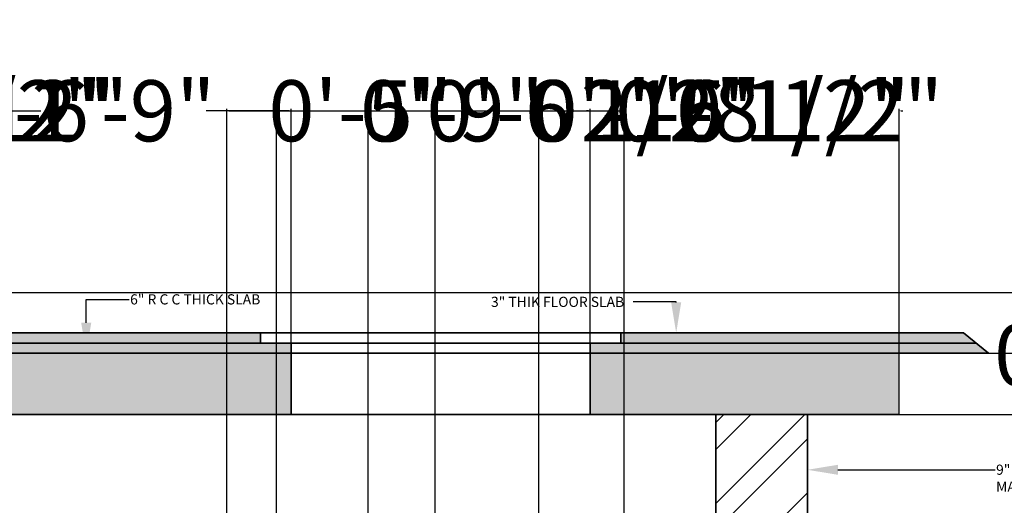
# Model space of a CAD drawing. Units: inches. Extents: x -34 to 285, y -151 to 155.
# Tile 8 of 10: x 129 to 225, y -58 to -10. Entities that reach past the tile are written whole.
import ezdxf
from ezdxf import colors
from ezdxf.entities.mleader import LeaderData, LeaderLine
from ezdxf.math import Vec2, Vec3

# ---------------------------------------------------------------- set-up
doc = ezdxf.new("R2010")
doc.units = ezdxf.units.IN
doc.header["$MEASUREMENT"] = 0
doc.linetypes.add('DASHED', pattern=[19.05, 12.7, -6.35])
for name, color, linetype, lineweight in [('A-ANNO-DIMS', 2, 'Continuous', 18), ('A-ANNO-TEXT', 7, 'Continuous', 25), ('A-DETL', 7, 'Continuous', 35), ('A-DETL-HIDN', 8, 'DASHED', 18), ('A-DETL-PATT', 8, 'Continuous', 18)]:
    doc.layers.add(name, color=color, linetype=linetype, lineweight=lineweight)
doc.styles.get("Standard").update_dxf_attribs({"font": 'arial.ttf'})
doc.dimstyles.get("Standard").update_dxf_attribs({"dimtxt": 6, "dimasz": 0.18, "dimexe": 0.18, "dimexo": 0.0625, "dimgap": 0.09, "dimtad": 0, "dimtih": 1, "dimtoh": 1, "dimzin": 0, "dimdsep": 46, "dimlunit": 3, "dimtxsty": 'Standard', "dimcen": 0.09, "dimadec": 0, "dimazin": 0, "dimtfac": 1, "dimtofl": 0, "dimtmove": 0, "dimatfit": 3, "dimfxl": 1, "dimtolj": 1, "dimtzin": 0, "dimarcsym": 0})

# ---------------------------------------------------------------- blocks, each defined once
blk = doc.blocks.new('*D53')
at = {"layer": 'A-ANNO-DIMS', "color": 0, "lineweight": -2, "transparency": 16777216}
for p, q in [((122.241, -48.906), (122.241, -18.978)), ((122.421, -19.158), (130.582, -19.158)), ((154.976, -19.158), (146.814, -19.158)), ((155.156, -48.906), (155.156, -18.978))]:
    blk.add_line(p, q, dxfattribs=at)
at = {"layer": 'A-ANNO-DIMS', "color": 0, "transparency": 16777216}
for points in [[(122.421, -19.128), (122.421, -19.188), (122.241, -19.158)], [(154.976, -19.128), (154.976, -19.188), (155.156, -19.158)]]:
    blk.add_solid(points, dxfattribs=at)
at = {"layer": 'Defpoints', "color": 0, "transparency": 16777216}
for p in [(155.156, -19.158), (122.241, -48.969), (155.156, -48.969)]:
    blk.add_point(p, dxfattribs=at)
at = {"layer": 'A-ANNO-DIMS', "color": 0, "transparency": 16777216, "insert": (138.698, -19.158), "char_height": 6, "attachment_point": 5}
blk.add_mtext('\\A1;2\'-9"', dxfattribs=at)
blk = doc.blocks.new('*D54')
at = {"layer": 'A-ANNO-DIMS', "color": 0, "lineweight": -2, "transparency": 16777216}
for p, q in [((155.156, -48.906), (155.156, -18.978)), ((155.336, -19.158), (184.338, -19.158)), ((184.518, -48.906), (184.518, -18.978)), ((184.518, -19.158), (184.698, -19.158))]:
    blk.add_line(p, q, dxfattribs=at)
at = {"layer": 'A-ANNO-DIMS', "color": 0, "transparency": 16777216}
for points in [[(155.336, -19.128), (155.336, -19.188), (155.156, -19.158)], [(184.338, -19.128), (184.338, -19.188), (184.518, -19.158)]]:
    blk.add_solid(points, dxfattribs=at)
at = {"layer": 'Defpoints', "color": 0, "transparency": 16777216}
for p in [(184.518, -19.158), (155.156, -48.969), (184.518, -48.969)]:
    blk.add_point(p, dxfattribs=at)
at = {"layer": 'A-ANNO-DIMS', "color": 0, "transparency": 16777216, "insert": (199.804, -19.158), "char_height": 6, "attachment_point": 5}
blk.add_mtext('\\A1;2\'-5 1/2"', dxfattribs=at)
blk = doc.blocks.new('*D55')
at = {"layer": 'A-ANNO-DIMS', "color": 0, "lineweight": -2, "transparency": 16777216}
for p, q in [((184.337711, -19.158499), (184.157711, -19.158499)), ((184.517711, -48.906465), (184.517711, -18.978499)), ((214.845773, -48.906465), (214.845773, -18.978499)), ((215.025773, -19.158499), (215.205773, -19.158499))]:
    blk.add_line(p, q, dxfattribs=at)
at = {"layer": 'A-ANNO-DIMS', "color": 0, "transparency": 16777216}
for points in [[(184.337711, -19.128499), (184.337711, -19.188499), (184.517711, -19.158499)], [(215.025773, -19.128499), (215.025773, -19.188499), (214.845773, -19.158499)]]:
    blk.add_solid(points, dxfattribs=at)
at = {"layer": 'Defpoints', "color": 0, "transparency": 16777216}
for p in [(214.845773, -19.158499), (184.517711, -48.968965), (214.845773, -48.968965)]:
    blk.add_point(p, dxfattribs=at)
at = {"layer": 'A-ANNO-DIMS', "color": 0, "transparency": 16777216, "insert": (199.681742, -19.158499), "char_height": 6, "attachment_point": 5}
blk.add_mtext('\\A1;2\'-6 1/2"', dxfattribs=at)
blk = doc.blocks.new('*D56')
at = {"layer": 'A-ANNO-DIMS', "color": 0, "lineweight": -2, "transparency": 16777216}
for p, q in [((46.493, -37.008), (241.637, -37.008)), ((241.457, -37.188), (241.457, -42.789)), ((46.493, -42.969), (241.637, -42.969)), ((241.457, -43.149), (241.277, -43.149)), ((241.457, -42.969), (241.457, -43.149))]:
    blk.add_line(p, q, dxfattribs=at)
at = {"layer": 'A-ANNO-DIMS', "color": 0, "transparency": 16777216}
for points in [[(241.427, -37.188), (241.487, -37.188), (241.457, -37.008)], [(241.427, -42.789), (241.487, -42.789), (241.457, -42.969)]]:
    blk.add_solid(points, dxfattribs=at)
at = {"layer": 'Defpoints', "color": 0, "transparency": 16777216}
for p in [(46.43, -37.008), (46.43, -42.969), (241.457, -42.969)]:
    blk.add_point(p, dxfattribs=at)
at = {"layer": 'A-ANNO-DIMS', "color": 0, "transparency": 16777216, "insert": (233.213, -43.149), "char_height": 6, "attachment_point": 5}
blk.add_mtext('\\A1;0\'-6"', dxfattribs=at)
blk = doc.blocks.new('*D59')
at = {"layer": 'A-ANNO-DIMS', "color": 0, "lineweight": -2, "transparency": 16777216}
for p, q in [((83.148, -48.969), (241.637, -48.969)), ((241.457, -49.149), (241.457, -52)), ((241.457, -61.235), (241.457, -58.384)), ((89.009, -61.415), (241.637, -61.415))]:
    blk.add_line(p, q, dxfattribs=at)
at = {"layer": 'A-ANNO-DIMS', "color": 0, "transparency": 16777216}
for points in [[(241.427, -49.149), (241.487, -49.149), (241.457, -48.969)], [(241.427, -61.235), (241.487, -61.235), (241.457, -61.415)]]:
    blk.add_solid(points, dxfattribs=at)
at = {"layer": 'Defpoints', "color": 0, "transparency": 16777216}
for p in [(83.086, -48.969), (88.947, -61.415), (241.457, -61.415)]:
    blk.add_point(p, dxfattribs=at)
at = {"layer": 'A-ANNO-DIMS', "color": 0, "transparency": 16777216, "insert": (241.457, -55.192), "char_height": 6, "attachment_point": 5}
blk.add_mtext('\\A1;1\'-0 1/2"', dxfattribs=at)
blk = doc.blocks.new('*D61')
at = {"layer": 'A-ANNO-DIMS', "color": 0, "lineweight": -2, "transparency": 16777216}
for p, q in [((148.846, -59.906), (148.846, -18.978)), ((149.026, -19.158), (153.535, -19.158)), ((153.715, -61.389), (153.715, -18.978)), ((153.715, -19.158), (153.895, -19.158))]:
    blk.add_line(p, q, dxfattribs=at)
at = {"layer": 'A-ANNO-DIMS', "color": 0, "transparency": 16777216}
for points in [[(149.026, -19.128), (149.026, -19.188), (148.846, -19.158)], [(153.535, -19.128), (153.535, -19.188), (153.715, -19.158)]]:
    blk.add_solid(points, dxfattribs=at)
at = {"layer": 'Defpoints', "color": 0, "transparency": 16777216}
for p in [(153.715, -19.158), (148.846, -59.969), (153.715, -61.451)]:
    blk.add_point(p, dxfattribs=at)
at = {"layer": 'A-ANNO-DIMS', "color": 0, "transparency": 16777216, "insert": (161.96, -19.158), "char_height": 6, "attachment_point": 5}
blk.add_mtext('\\A1;0\'-5"', dxfattribs=at)
blk = doc.blocks.new('*D62')
at = {"layer": 'A-ANNO-DIMS', "color": 0, "lineweight": -2, "transparency": 16777216}
for p, q in [((155.218, -48.969), (241.637, -48.969)), ((241.457, -49.149), (241.457, -52.018)), ((241.457, -61.271), (241.457, -58.402)), ((153.777, -61.451), (241.637, -61.451))]:
    blk.add_line(p, q, dxfattribs=at)
at = {"layer": 'A-ANNO-DIMS', "color": 0, "transparency": 16777216}
for points in [[(241.427, -49.149), (241.487, -49.149), (241.457, -48.969)], [(241.427, -61.271), (241.487, -61.271), (241.457, -61.451)]]:
    blk.add_solid(points, dxfattribs=at)
at = {"layer": 'Defpoints', "color": 0, "transparency": 16777216}
for p in [(155.156, -48.969), (153.715, -61.451), (241.457, -61.451)]:
    blk.add_point(p, dxfattribs=at)
at = {"layer": 'A-ANNO-DIMS', "color": 0, "transparency": 16777216, "insert": (241.457, -55.21), "char_height": 6, "attachment_point": 5}
blk.add_mtext('\\A1;1\'-0 1/2"', dxfattribs=at)
blk = doc.blocks.new('*D69')
at = {"layer": 'A-ANNO-DIMS', "color": 0, "lineweight": -2, "transparency": 16777216}
for p, q in [((97.668, -81.282), (97.668, -18.978)), ((97.848, -19.158), (105.119, -19.158)), ((105.299, -90.467), (105.299, -18.978)), ((105.299, -19.158), (105.479, -19.158))]:
    blk.add_line(p, q, dxfattribs=at)
at = {"layer": 'A-ANNO-DIMS', "color": 0, "transparency": 16777216}
for points in [[(97.848, -19.128), (97.848, -19.188), (97.668, -19.158)], [(105.119, -19.128), (105.119, -19.188), (105.299, -19.158)]]:
    blk.add_solid(points, dxfattribs=at)
at = {"layer": 'Defpoints', "color": 0, "transparency": 16777216}
for p in [(105.299, -19.158), (97.668, -81.345), (105.299, -90.53)]:
    blk.add_point(p, dxfattribs=at)
at = {"layer": 'A-ANNO-DIMS', "color": 0, "transparency": 16777216, "insert": (120.534, -19.158), "char_height": 6, "attachment_point": 5}
blk.add_mtext('\\A1;0\'-7 1/2"', dxfattribs=at)
blk = doc.blocks.new('*D70')
at = {"layer": 'A-ANNO-DIMS', "color": 0, "lineweight": -2, "transparency": 16777216}
for p, q in [((105.299, -90.467), (105.299, -18.978)), ((105.479, -19.158), (115.871, -19.158)), ((116.051, -97.053), (116.051, -18.978)), ((116.051, -19.158), (116.231, -19.158))]:
    blk.add_line(p, q, dxfattribs=at)
at = {"layer": 'A-ANNO-DIMS', "color": 0, "transparency": 16777216}
for points in [[(105.479, -19.128), (105.479, -19.188), (105.299, -19.158)], [(115.871, -19.128), (115.871, -19.188), (116.051, -19.158)]]:
    blk.add_solid(points, dxfattribs=at)
at = {"layer": 'Defpoints', "color": 0, "transparency": 16777216}
for p in [(116.051, -19.158), (105.299, -90.53), (116.051, -97.116)]:
    blk.add_point(p, dxfattribs=at)
at = {"layer": 'A-ANNO-DIMS', "color": 0, "transparency": 16777216, "insert": (126.627, -19.158), "char_height": 6, "attachment_point": 5}
blk.add_mtext('\\A1;0\'-11"', dxfattribs=at)
blk = doc.blocks.new('*D71')
at = {"layer": 'A-ANNO-DIMS', "color": 0, "lineweight": -2, "transparency": 16777216}
for p, q in [((116.051, -97.053), (116.051, -18.978)), ((116.231, -19.158), (121.719, -19.158)), ((121.899, -103.966), (121.899, -18.978)), ((121.899, -19.158), (122.079, -19.158))]:
    blk.add_line(p, q, dxfattribs=at)
at = {"layer": 'A-ANNO-DIMS', "color": 0, "transparency": 16777216}
for points in [[(116.231, -19.128), (116.231, -19.188), (116.051, -19.158)], [(121.719, -19.128), (121.719, -19.188), (121.899, -19.158)]]:
    blk.add_solid(points, dxfattribs=at)
at = {"layer": 'Defpoints', "color": 0, "transparency": 16777216}
for p in [(121.899, -19.158), (116.051, -97.116), (121.899, -104.028)]:
    blk.add_point(p, dxfattribs=at)
at = {"layer": 'A-ANNO-DIMS', "color": 0, "transparency": 16777216, "insert": (130.144, -19.158), "char_height": 6, "attachment_point": 5}
blk.add_mtext('\\A1;0\'-6"', dxfattribs=at)
blk = doc.blocks.new('*D79')
at = {"layer": 'A-ANNO-DIMS', "color": 0, "lineweight": -2, "transparency": 16777216}
for p, q in [((153.715, -61.389), (153.715, -18.978)), ((153.895, -19.158), (162.535, -19.158)), ((162.715, -73.74), (162.715, -18.978)), ((162.715, -19.158), (162.895, -19.158))]:
    blk.add_line(p, q, dxfattribs=at)
at = {"layer": 'A-ANNO-DIMS', "color": 0, "transparency": 16777216}
for points in [[(153.895, -19.128), (153.895, -19.188), (153.715, -19.158)], [(162.535, -19.128), (162.535, -19.188), (162.715, -19.158)]]:
    blk.add_solid(points, dxfattribs=at)
at = {"layer": 'Defpoints', "color": 0, "transparency": 16777216}
for p in [(162.715, -19.158), (153.715, -61.451), (162.715, -73.803)]:
    blk.add_point(p, dxfattribs=at)
at = {"layer": 'A-ANNO-DIMS', "color": 0, "transparency": 16777216, "insert": (170.96, -19.158), "char_height": 6, "attachment_point": 5}
blk.add_mtext('\\A1;0\'-9"', dxfattribs=at)
blk = doc.blocks.new('*D80')
at = {"layer": 'A-ANNO-DIMS', "color": 0, "lineweight": -2, "transparency": 16777216}
for p, q in [((162.715, -73.74), (162.715, -18.978)), ((162.895, -19.158), (169.123, -19.158)), ((169.303, -84.63), (169.303, -18.978)), ((169.303, -19.158), (169.483, -19.158))]:
    blk.add_line(p, q, dxfattribs=at)
at = {"layer": 'A-ANNO-DIMS', "color": 0, "transparency": 16777216}
for points in [[(162.895, -19.128), (162.895, -19.188), (162.715, -19.158)], [(169.123, -19.128), (169.123, -19.188), (169.303, -19.158)]]:
    blk.add_solid(points, dxfattribs=at)
at = {"layer": 'Defpoints', "color": 0, "transparency": 16777216}
for p in [(169.303, -19.158), (162.715, -73.803), (169.303, -84.693)]:
    blk.add_point(p, dxfattribs=at)
at = {"layer": 'A-ANNO-DIMS', "color": 0, "transparency": 16777216, "insert": (184.538, -19.158), "char_height": 6, "attachment_point": 5}
blk.add_mtext('\\A1;0\'-6 1/2"', dxfattribs=at)
blk = doc.blocks.new('*D81')
at = {"layer": 'A-ANNO-DIMS', "color": 0, "lineweight": -2, "transparency": 16777216}
for p, q in [((169.303, -84.63), (169.303, -18.978)), ((169.483, -19.158), (179.302, -19.158)), ((179.482, -96.63), (179.482, -18.978)), ((179.482, -19.158), (179.662, -19.158))]:
    blk.add_line(p, q, dxfattribs=at)
at = {"layer": 'A-ANNO-DIMS', "color": 0, "transparency": 16777216}
for points in [[(169.483, -19.128), (169.483, -19.188), (169.303, -19.158)], [(179.302, -19.128), (179.302, -19.188), (179.482, -19.158)]]:
    blk.add_solid(points, dxfattribs=at)
at = {"layer": 'Defpoints', "color": 0, "transparency": 16777216}
for p in [(179.482, -19.158), (169.303, -84.693), (179.482, -96.693)]:
    blk.add_point(p, dxfattribs=at)
at = {"layer": 'A-ANNO-DIMS', "color": 0, "transparency": 16777216, "insert": (190.057, -19.158), "char_height": 6, "attachment_point": 5}
blk.add_mtext('\\A1;0\'-10"', dxfattribs=at)
blk = doc.blocks.new('*D82')
at = {"layer": 'A-ANNO-DIMS', "color": 0, "lineweight": -2, "transparency": 16777216}
for p, q in [((179.482, -96.63), (179.482, -18.978)), ((179.662, -19.158), (187.666, -19.158)), ((187.846, -108.007), (187.846, -18.978)), ((187.846, -19.158), (188.026, -19.158))]:
    blk.add_line(p, q, dxfattribs=at)
at = {"layer": 'A-ANNO-DIMS', "color": 0, "transparency": 16777216}
for points in [[(179.662, -19.128), (179.662, -19.188), (179.482, -19.158)], [(187.666, -19.128), (187.666, -19.188), (187.846, -19.158)]]:
    blk.add_solid(points, dxfattribs=at)
at = {"layer": 'Defpoints', "color": 0, "transparency": 16777216}
for p in [(187.846, -19.158), (179.482, -96.693), (187.846, -108.07)]:
    blk.add_point(p, dxfattribs=at)
at = {"layer": 'A-ANNO-DIMS', "color": 0, "transparency": 16777216, "insert": (203.081, -19.158), "char_height": 6, "attachment_point": 5}
blk.add_mtext('\\A1;0\'-8 1/2"', dxfattribs=at)

msp = doc.modelspace()

# ---------------------------------------------------------------- hatches: boundary and pattern name
at = {"layer": 'A-DETL-PATT'}
h = msp.add_hatch(dxfattribs=at)
h.set_pattern_fill('AR-SAND', color=256, scale=0.1)
h.paths.add_polyline_path([(152.156, -40.969), (125.241, -40.969), (125.241, -41.969), (152.156, -41.969)])
h.paths.add_polyline_path([(155.156, -41.969), (152.156, -41.969), (122.241, -41.969), (122.241, -42.969), (155.156, -42.969)])
h = msp.add_hatch(dxfattribs=at)
h.set_pattern_fill('AR-SAND', color=256, scale=0.1)
h.set_pattern_definition([(37.5, (0, 0), (-0.00629934, 0.19268238), [0, -0.152, 0, -0.17, 0, -0.1625]), (7.5, (0, 0), (0.17697767, 0.2822146), [0, -0.082, 0, -0.137, 0, -0.0525]), (327.5, (-0.123, 0), (0.31141419, 0.0005659), [0, -0.05, 0, -0.18, 0, -0.235]), (317.5, (-0.123, 0), (0.30061266, 0.08776756), [0, -0.025, 0, -0.118, 0, -0.135])])
h.paths.add_polyline_path([(221.174, -40.969), (187.518, -40.969), (187.518, -41.969), (222.391, -41.969)])
h.paths.add_polyline_path([(222.391, -41.969), (187.518, -41.969), (184.518, -41.969), (184.518, -42.969), (214.846, -42.969), (223.607, -42.969)])
h = msp.add_hatch(dxfattribs=at)
h.set_pattern_fill('AR-CONC', color=256, scale=0.4)
h.set_pattern_definition([(50, (0, 0), (2.86904, -0.251009), [0.3, -3.3]), (355, (0, 0), (-0.555005, 3.00877), [0.24, -2.64]), (100.4514, (0.239, -0.021), (2.314035, 2.75776), [0.25496, -2.80457]), (46.1842, (0, 0.8), (4.268965, -0.662077), [0.45, -4.95]), (96.6356, (0.3557, 0.745), (3.73865, 3.896474), [0.38244, -4.206855]), (351.1842, (0, 0.8), (3.73865, 3.896474), [0.36, -3.96]), (21, (0.4, 0.6), (2.387628, -1.610476), [0.3, -3.3]), (326, (0.4, 0.6), (0.97326, 2.9006), [0.24, -2.64]), (71.4514, (0.599, 0.4658), (3.36089, 1.290125), [0.25496, -2.80457]), (37.5, (0, 0), (0.0486394, 1.3315754), [0, -2.608, 0, -2.68, 0, -2.65]), (7.5, (0, 0), (1.052278, 1.577647), [0, -1.528, 0, -2.548, 0, -1.01]), (327.5, (-0.892, 0), (2.1352897, -0.0902195), [0, -1, 0, -3.12, 0, -4.14]), (317.5, (-1.292, 0), (2.332745, 0.40042), [0, -1.3, 0, -2.072, 0, -2.94])])
h.paths.add_polyline_path([(214.846, -48.969), (214.846, -42.969), (184.518, -42.969), (184.518, -48.969)])
h.paths.add_polyline_path([(122.241, -42.969), (122.241, -48.969), (155.156, -48.969), (155.156, -42.969)])
h.paths.add_polyline_path([(214.846, -114.969), (22.846, -114.969), (22.846, -120.969), (214.846, -120.969)])
h = msp.add_hatch(dxfattribs=at)
h.set_pattern_fill('ANSI32', color=256, scale=15)
h.paths.add_polyline_path([(205.846, -48.969), (196.846, -48.969), (196.846, -63.469), (205.846, -63.469)])

# ---------------------------------------------------------------- linework, layer by layer
at = {"layer": 'A-DETL'}
for p, q in [((46.43, -40.969), (221.174, -40.969)), ((152.156, -41.969), (152.156, -40.969)), ((187.518, -41.969), (187.518, -40.969)), ((223.607, -42.969), (221.174, -40.969)), ((46.43, -41.969), (222.391, -41.969)), ((155.156, -41.969), (152.156, -41.969)), ((155.156, -42.969), (155.156, -41.969)), ((184.518, -42.969), (184.518, -41.969)), ((184.518, -41.969), (187.518, -41.969)), ((46.43, -42.969), (214.846, -42.969)), ((46.43, -42.969), (205.846, -42.969)), ((155.156, -48.969), (155.156, -42.969)), ((184.518, -42.969), (184.518, -48.969)), ((214.846, -42.969), (223.607, -42.969)), ((22.846, -48.969), (214.846, -48.969)), ((196.846, -48.969), (196.846, -114.969)), ((205.846, -48.969), (205.846, -114.969))]:
    msp.add_line(p, q, dxfattribs=at)
at = {"layer": 'A-DETL-HIDN'}
msp.add_line((214.846, -42.969), (214.846, -48.969), dxfattribs=at)

# ---------------------------------------------------------------- dimensions: what is measured, and where the dimension line sits
at = {"layer": 'A-ANNO-DIMS'}
for base, p1, p2, picture, middle in [((105.299, -19.158), (97.668, -81.345), (105.299, -90.53), '*D69', (120.534, -19.158)), ((184.518, -19.158), (155.156, -48.969), (184.518, -48.969), '*D54', (199.804, -19.158)), ((169.303, -19.158), (162.715, -73.803), (169.303, -84.693), '*D80', (184.538, -19.158)), ((187.846, -19.158), (179.482, -96.693), (187.846, -108.07), '*D82', (203.081, -19.158)), ((214.846, -19.158), (184.518, -48.969), (214.846, -48.969), '*D55', (199.682, -19.158)), ((116.051, -19.158), (105.299, -90.53), (116.051, -97.116), '*D70', (126.627, -19.158)), ((121.899, -19.158), (116.051, -97.116), (121.899, -104.028), '*D71', (130.144, -19.158)), ((155.156, -19.158), (122.241, -48.969), (155.156, -48.969), '*D53', (138.698, -19.158)), ((153.715, -19.158), (148.846, -59.969), (153.715, -61.451), '*D61', (161.96, -19.158)), ((162.715, -19.158), (153.715, -61.451), (162.715, -73.803), '*D79', (170.96, -19.158)), ((179.482, -19.158), (169.303, -84.693), (179.482, -96.693), '*D81', (190.057, -19.158))]:
    dim = msp.add_linear_dim(base=base, p1=p1, p2=p2, dimstyle='Standard', override={"dimdec": 1, "dimlfac": 1, "dimrnd": 0, "dimzin": 1, "dimdsep": 46, "dimlunit": 4, "dimfrac": 2}, dxfattribs=at)
    dim.commit()
    dim.dimension.update_dxf_attribs({"geometry": picture, "text_midpoint": middle})
for base, p1, p2, picture, middle in [((241.457, -42.969), (46.43, -37.008), (46.43, -42.969), '*D56', (233.213, -43.149)), ((241.457, -61.415), (83.086, -48.969), (88.947, -61.415), '*D59', (241.457, -55.192)), ((241.457, -61.451), (155.156, -48.969), (153.715, -61.451), '*D62', (241.457, -55.21))]:
    dim = msp.add_linear_dim(base=base, p1=p1, p2=p2, angle=90, dimstyle='Standard', override={"dimdec": 1, "dimlfac": 1, "dimrnd": 0, "dimzin": 1, "dimdsep": 46, "dimlunit": 4, "dimfrac": 2}, dxfattribs=at)
    dim.commit()
    dim.dimension.update_dxf_attribs({"geometry": picture, "text_midpoint": middle})

# ---------------------------------------------------------------- leaders
at = {"layer": 'A-ANNO-TEXT'}
ml = msp.add_multileader_mtext('Standard', dxfattribs=at)
ml.set_content('6" R C C THICK SLAB', color=(248, 215, 49))
ml.set_leader_properties()
ml.build(insert=Vec2(0, 0))
ml.multileader.update_dxf_attribs({"dogleg_length": 4.22, "arrow_head_size": 3})
ctx = ml.context
ctx.base_point, ctx.char_height, ctx.arrow_head_size, ctx.landing_gap_size, ctx.plane_origin = Vec3(139.261, -37.683), 1, 3, 0.09, Vec3(135.041, -42.969)
notes = []
notes.append((ctx, [(0, (1, 1, 0), (135.041, -37.683), (1, 0), 4.22, [(0, [(135.041, -42.969)], 0, [])])]))
ctx.mtext.insert, ctx.mtext.flow_direction = Vec3(139.351, -37.175), 5
ml = msp.add_multileader_mtext('Standard', dxfattribs=at)
ml.set_content('3" THIK FLOOR SLAB', color=(248, 215, 49))
ml.set_leader_properties()
ml.build(insert=Vec2(0, 0))
ml.multileader.update_dxf_attribs({"dogleg_length": 4.22, "arrow_head_size": 3})
ctx = ml.context
ctx.base_point, ctx.char_height, ctx.arrow_head_size, ctx.landing_gap_size, ctx.plane_origin = Vec3(174.689, -37.93), 1, 3, 0.09, Vec3(192.96, -40.969)
notes.append((ctx, [(0, (1, 1, 0), (192.96, -37.93), (-1, 0), 4.22, [(0, [(192.96, -40.969)], 0, [])])]))
ctx.mtext.insert, ctx.mtext.flow_direction = Vec3(174.779, -37.421), 5
ml = msp.add_multileader_mtext('Standard', dxfattribs=at)
ml.set_content('9" THICK BRICK \\PMASONRY ', color=(248, 215, 49))
ml.set_leader_properties()
ml.build(insert=Vec2(0, 0))
ml.multileader.update_dxf_attribs({"dogleg_length": 4.22, "arrow_head_size": 3})
ctx = ml.context
ctx.base_point, ctx.char_height, ctx.arrow_head_size, ctx.landing_gap_size, ctx.plane_origin = Vec3(224.277, -54.411), 1, 3, 0.09, Vec3(205.846, -54.411)
notes.append((ctx, [(0, (1, 1, 0), (220.057, -54.411), (1, 0), 4.22, [(0, [(205.846, -54.411)], 0, [])])]))
ctx.mtext.insert, ctx.mtext.flow_direction = Vec3(224.367, -53.902), 5
for ctx, leaders in notes:
    for number, flags, end, landing, length, lines in leaders:
        leader = LeaderData()
        leader.index, (leader.has_last_leader_line, leader.has_dogleg_vector, leader.attachment_direction) = number, flags
        leader.last_leader_point, leader.dogleg_vector, leader.dogleg_length = Vec3(end), Vec3(landing), length
        for number, points, colour, breaks in lines:
            line = LeaderLine()
            line.index, line.vertices, line.color, line.breaks = number, Vec3.list(points), colors.encode_raw_color(colour), breaks
            leader.lines.append(line)
        ctx.leaders.append(leader)

doc.saveas('drawing.dxf')
